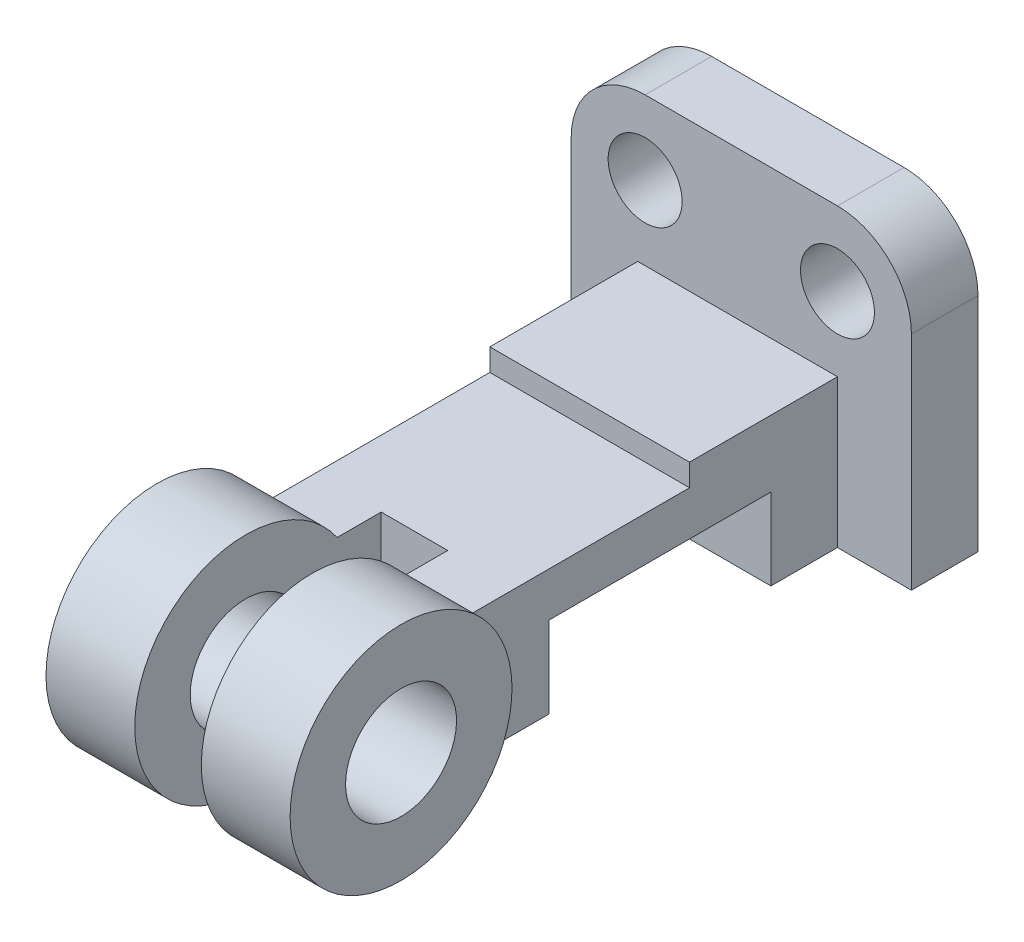
ISO-10303-21;
HEADER;
FILE_DESCRIPTION(('STEP AP214'),'2;1');
FILE_NAME('part.step','',(''),(''),'','','');
FILE_SCHEMA(('AUTOMOTIVE_DESIGN { 1 0 10303 214 1 1 1 1 }'));
ENDSEC;
DATA;
#1=APPLICATION_CONTEXT('core data for automotive mechanical design processes');
#2=APPLICATION_PROTOCOL_DEFINITION('international standard','automotive_design',2000,#1);
#3=PRODUCT_CONTEXT('',#1,'mechanical');
#4=PRODUCT('Part','Part','',(#3));
#5=PRODUCT_RELATED_PRODUCT_CATEGORY('part','',(#4));
#6=PRODUCT_DEFINITION_FORMATION('','',#4);
#7=PRODUCT_DEFINITION_CONTEXT('part definition',#1,'design');
#8=PRODUCT_DEFINITION('design','',#6,#7);
#9=PRODUCT_DEFINITION_SHAPE('','',#8);
#10=(LENGTH_UNIT() NAMED_UNIT(*) SI_UNIT(.MILLI.,.METRE.));
#11=(NAMED_UNIT(*) PLANE_ANGLE_UNIT() SI_UNIT($,.RADIAN.));
#12=(NAMED_UNIT(*) SI_UNIT($,.STERADIAN.) SOLID_ANGLE_UNIT());
#13=UNCERTAINTY_MEASURE_WITH_UNIT(LENGTH_MEASURE(1.E-05),#10,'distance_accuracy_value','');
#14=(GEOMETRIC_REPRESENTATION_CONTEXT(3) GLOBAL_UNCERTAINTY_ASSIGNED_CONTEXT((#13)) GLOBAL_UNIT_ASSIGNED_CONTEXT((#10,
#11,#12)) REPRESENTATION_CONTEXT('',''));
#15=CARTESIAN_POINT('',(0.,0.,0.));
#16=DIRECTION('',(0.,0.,1.));
#17=DIRECTION('',(1.,0.,0.));
#18=AXIS2_PLACEMENT_3D('',#15,#16,#17);
#19=CARTESIAN_POINT('',(78.,17.,142.));
#20=DIRECTION('',(-1.,0.,0.));
#21=DIRECTION('',(0.,-1.,0.));
#22=AXIS2_PLACEMENT_3D('',#19,#20,#21);
#23=CYLINDRICAL_SURFACE('',#22,30.);
#24=CARTESIAN_POINT('',(78.,17.,142.));
#25=DIRECTION('',(1.,0.,0.));
#26=DIRECTION('',(0.,1.,0.));
#27=AXIS2_PLACEMENT_3D('',#24,#25,#26);
#28=CIRCLE('',#27,30.);
#29=CARTESIAN_POINT('',(78.,47.,142.));
#30=VERTEX_POINT('',#29);
#31=EDGE_CURVE('E224',#30,#30,#28,.T.);
#32=ORIENTED_EDGE('',*,*,#31,.F.);
#33=EDGE_LOOP('',(#32));
#34=FACE_BOUND('',#33,.T.);
#35=CARTESIAN_POINT('',(54.,17.,142.));
#36=DIRECTION('',(-1.,0.,0.));
#37=DIRECTION('',(0.,0.,1.));
#38=AXIS2_PLACEMENT_3D('',#35,#36,#37);
#39=CIRCLE('',#38,30.);
#40=CARTESIAN_POINT('',(54.,0.,117.281585811383));
#41=VERTEX_POINT('',#40);
#42=CARTESIAN_POINT('',(54.,34.,117.281585811383));
#43=VERTEX_POINT('',#42);
#44=EDGE_CURVE('E187',#41,#43,#39,.T.);
#45=ORIENTED_EDGE('',*,*,#44,.F.);
#46=DIRECTION('',(-1.,0.,0.));
#47=VECTOR('',#46,1.);
#48=CARTESIAN_POINT('',(78.,0.,117.281585811383));
#49=LINE('',#48,#47);
#50=CARTESIAN_POINT('',(72.,0.,117.281585811383));
#51=VERTEX_POINT('',#50);
#52=EDGE_CURVE('E233',#41,#51,#49,.F.);
#53=ORIENTED_EDGE('',*,*,#52,.T.);
#54=CARTESIAN_POINT('',(72.,17.,142.));
#55=DIRECTION('',(1.,0.,0.));
#56=DIRECTION('',(0.,1.,0.));
#57=AXIS2_PLACEMENT_3D('',#54,#55,#56);
#58=CIRCLE('',#57,30.);
#59=CARTESIAN_POINT('',(72.,34.,117.281585811383));
#60=VERTEX_POINT('',#59);
#61=EDGE_CURVE('E193',#60,#51,#58,.F.);
#62=ORIENTED_EDGE('',*,*,#61,.F.);
#63=DIRECTION('',(-1.,0.,0.));
#64=VECTOR('',#63,1.);
#65=CARTESIAN_POINT('',(78.,34.,117.281585811383));
#66=LINE('',#65,#64);
#67=EDGE_CURVE('E48',#43,#60,#66,.F.);
#68=ORIENTED_EDGE('',*,*,#67,.F.);
#69=EDGE_LOOP('',(#45,#53,#62,#68));
#70=FACE_BOUND('',#69,.T.);
#71=ADVANCED_FACE('F39',(#34,#70),#23,.T.);
#72=CARTESIAN_POINT('',(78.,17.,142.));
#73=DIRECTION('',(-1.,0.,0.));
#74=DIRECTION('',(0.,-1.,0.));
#75=AXIS2_PLACEMENT_3D('',#72,#73,#74);
#76=CYLINDRICAL_SURFACE('',#75,15.);
#77=CARTESIAN_POINT('',(78.,17.,142.));
#78=DIRECTION('',(1.,0.,0.));
#79=DIRECTION('',(0.,1.,0.));
#80=AXIS2_PLACEMENT_3D('',#77,#78,#79);
#81=CIRCLE('',#80,15.);
#82=CARTESIAN_POINT('',(78.,32.,142.));
#83=VERTEX_POINT('',#82);
#84=EDGE_CURVE('E225',#83,#83,#81,.T.);
#85=ORIENTED_EDGE('',*,*,#84,.T.);
#86=EDGE_LOOP('',(#85));
#87=FACE_BOUND('',#86,.T.);
#88=CARTESIAN_POINT('',(54.,17.,142.));
#89=DIRECTION('',(-1.,0.,0.));
#90=DIRECTION('',(0.,0.,1.));
#91=AXIS2_PLACEMENT_3D('',#88,#89,#90);
#92=CIRCLE('',#91,15.);
#93=CARTESIAN_POINT('',(54.,17.,157.));
#94=VERTEX_POINT('',#93);
#95=EDGE_CURVE('E195',#94,#94,#92,.T.);
#96=ORIENTED_EDGE('',*,*,#95,.T.);
#97=EDGE_LOOP('',(#96));
#98=FACE_BOUND('',#97,.T.);
#99=ADVANCED_FACE('F413',(#87,#98),#76,.F.);
#100=CARTESIAN_POINT('',(0.,0.,18.));
#101=DIRECTION('',(0.,1.,0.));
#102=DIRECTION('',(0.,0.,1.));
#103=AXIS2_PLACEMENT_3D('',#100,#101,#102);
#104=PLANE('',#103);
#105=DIRECTION('',(-1.,0.,0.));
#106=VECTOR('',#105,1.);
#107=CARTESIAN_POINT('',(0.,0.,105.372540600415));
#108=LINE('',#107,#106);
#109=CARTESIAN_POINT('',(54.,0.,105.372540600415));
#110=VERTEX_POINT('',#109);
#111=CARTESIAN_POINT('',(36.,0.,105.372540600415));
#112=VERTEX_POINT('',#111);
#113=EDGE_CURVE('E201',#110,#112,#108,.T.);
#114=ORIENTED_EDGE('',*,*,#113,.T.);
#115=DIRECTION('',(0.,0.,1.));
#116=VECTOR('',#115,1.);
#117=CARTESIAN_POINT('',(36.,0.,18.));
#118=LINE('',#117,#116);
#119=CARTESIAN_POINT('',(36.,0.,117.281585811383));
#120=VERTEX_POINT('',#119);
#121=EDGE_CURVE('E210',#112,#120,#118,.T.);
#122=ORIENTED_EDGE('',*,*,#121,.T.);
#123=CARTESIAN_POINT('',(18.,0.,117.281585811383));
#124=VERTEX_POINT('',#123);
#125=EDGE_CURVE('E235',#124,#120,#49,.F.);
#126=ORIENTED_EDGE('',*,*,#125,.F.);
#127=DIRECTION('',(0.,0.,-1.));
#128=VECTOR('',#127,1.);
#129=CARTESIAN_POINT('',(18.,0.,18.));
#130=LINE('',#129,#128);
#131=CARTESIAN_POINT('',(18.,0.,96.));
#132=VERTEX_POINT('',#131);
#133=EDGE_CURVE('E278',#124,#132,#130,.T.);
#134=ORIENTED_EDGE('',*,*,#133,.T.);
#135=DIRECTION('',(1.,0.,0.));
#136=VECTOR('',#135,1.);
#137=CARTESIAN_POINT('',(18.,0.,96.));
#138=LINE('',#137,#136);
#139=CARTESIAN_POINT('',(72.,0.,96.));
#140=VERTEX_POINT('',#139);
#141=EDGE_CURVE('E260',#132,#140,#138,.T.);
#142=ORIENTED_EDGE('',*,*,#141,.T.);
#143=DIRECTION('',(0.,0.,-1.));
#144=VECTOR('',#143,1.);
#145=CARTESIAN_POINT('',(72.,0.,18.));
#146=LINE('',#145,#144);
#147=EDGE_CURVE('E271',#51,#140,#146,.T.);
#148=ORIENTED_EDGE('',*,*,#147,.F.);
#149=ORIENTED_EDGE('',*,*,#52,.F.);
#150=DIRECTION('',(0.,0.,-1.));
#151=VECTOR('',#150,1.);
#152=CARTESIAN_POINT('',(54.,0.,18.));
#153=LINE('',#152,#151);
#154=EDGE_CURVE('E186',#41,#110,#153,.T.);
#155=ORIENTED_EDGE('',*,*,#154,.T.);
#156=EDGE_LOOP('',(#114,#122,#126,#134,#142,#148,#149,#155));
#157=FACE_BOUND('',#156,.T.);
#158=ADVANCED_FACE('F419',(#157),#104,.F.);
#159=CARTESIAN_POINT('',(18.,34.,58.));
#160=DIRECTION('',(0.,1.,0.));
#161=DIRECTION('',(-1.,0.,0.));
#162=AXIS2_PLACEMENT_3D('',#159,#160,#161);
#163=PLANE('',#162);
#164=DIRECTION('',(0.,0.,1.));
#165=VECTOR('',#164,1.);
#166=CARTESIAN_POINT('',(36.,34.,117.281585811383));
#167=LINE('',#166,#165);
#168=CARTESIAN_POINT('',(36.,34.,105.372540600415));
#169=VERTEX_POINT('',#168);
#170=CARTESIAN_POINT('',(36.,34.,117.281585811383));
#171=VERTEX_POINT('',#170);
#172=EDGE_CURVE('E467',#169,#171,#167,.T.);
#173=ORIENTED_EDGE('',*,*,#172,.F.);
#174=DIRECTION('',(-1.,0.,0.));
#175=VECTOR('',#174,1.);
#176=CARTESIAN_POINT('',(54.,34.,105.372540600415));
#177=LINE('',#176,#175);
#178=CARTESIAN_POINT('',(54.,34.,105.372540600415));
#179=VERTEX_POINT('',#178);
#180=EDGE_CURVE('E181',#179,#169,#177,.T.);
#181=ORIENTED_EDGE('',*,*,#180,.F.);
#182=DIRECTION('',(0.,0.,-1.));
#183=VECTOR('',#182,1.);
#184=CARTESIAN_POINT('',(54.,34.,117.281585811383));
#185=LINE('',#184,#183);
#186=EDGE_CURVE('E176',#43,#179,#185,.T.);
#187=ORIENTED_EDGE('',*,*,#186,.F.);
#188=ORIENTED_EDGE('',*,*,#67,.T.);
#189=DIRECTION('',(0.,0.,1.));
#190=VECTOR('',#189,1.);
#191=CARTESIAN_POINT('',(72.,34.,58.));
#192=LINE('',#191,#190);
#193=CARTESIAN_POINT('',(72.,34.,58.));
#194=VERTEX_POINT('',#193);
#195=EDGE_CURVE('E251',#194,#60,#192,.T.);
#196=ORIENTED_EDGE('',*,*,#195,.F.);
#197=DIRECTION('',(1.,0.,0.));
#198=VECTOR('',#197,1.);
#199=CARTESIAN_POINT('',(18.,34.,58.));
#200=LINE('',#199,#198);
#201=CARTESIAN_POINT('',(18.,34.,58.));
#202=VERTEX_POINT('',#201);
#203=EDGE_CURVE('E265',#202,#194,#200,.T.);
#204=ORIENTED_EDGE('',*,*,#203,.F.);
#205=DIRECTION('',(0.,0.,1.));
#206=VECTOR('',#205,1.);
#207=CARTESIAN_POINT('',(18.,34.,58.));
#208=LINE('',#207,#206);
#209=CARTESIAN_POINT('',(18.,34.,117.281585811383));
#210=VERTEX_POINT('',#209);
#211=EDGE_CURVE('E263',#202,#210,#208,.T.);
#212=ORIENTED_EDGE('',*,*,#211,.T.);
#213=EDGE_CURVE('E11',#210,#171,#66,.F.);
#214=ORIENTED_EDGE('',*,*,#213,.T.);
#215=EDGE_LOOP('',(#173,#181,#187,#188,#196,#204,#212,#214));
#216=FACE_BOUND('',#215,.T.);
#217=ADVANCED_FACE('F177',(#216),#163,.T.);
#218=CARTESIAN_POINT('',(72.,0.,36.));
#219=VERTEX_POINT('',#218);
#220=CARTESIAN_POINT('',(72.,0.,18.));
#221=VERTEX_POINT('',#220);
#222=EDGE_CURVE('E289',#219,#221,#146,.T.);
#223=ORIENTED_EDGE('',*,*,#222,.F.);
#224=DIRECTION('',(1.,0.,0.));
#225=VECTOR('',#224,1.);
#226=CARTESIAN_POINT('',(18.,0.,36.));
#227=LINE('',#226,#225);
#228=CARTESIAN_POINT('',(18.,0.,36.));
#229=VERTEX_POINT('',#228);
#230=EDGE_CURVE('E253',#229,#219,#227,.T.);
#231=ORIENTED_EDGE('',*,*,#230,.F.);
#232=CARTESIAN_POINT('',(18.,0.,18.));
#233=VERTEX_POINT('',#232);
#234=EDGE_CURVE('E276',#229,#233,#130,.T.);
#235=ORIENTED_EDGE('',*,*,#234,.T.);
#236=DIRECTION('',(1.,0.,0.));
#237=VECTOR('',#236,1.);
#238=CARTESIAN_POINT('',(0.,0.,18.));
#239=LINE('',#238,#237);
#240=CARTESIAN_POINT('',(0.,0.,18.));
#241=VERTEX_POINT('',#240);
#242=EDGE_CURVE('E313',#241,#233,#239,.T.);
#243=ORIENTED_EDGE('',*,*,#242,.F.);
#244=DIRECTION('',(0.,0.,-1.));
#245=VECTOR('',#244,1.);
#246=CARTESIAN_POINT('',(0.,0.,18.));
#247=LINE('',#246,#245);
#248=CARTESIAN_POINT('',(0.,0.,0.));
#249=VERTEX_POINT('',#248);
#250=EDGE_CURVE('E199',#241,#249,#247,.T.);
#251=ORIENTED_EDGE('',*,*,#250,.T.);
#252=DIRECTION('',(1.,0.,0.));
#253=VECTOR('',#252,1.);
#254=CARTESIAN_POINT('',(0.,0.,0.));
#255=LINE('',#254,#253);
#256=CARTESIAN_POINT('',(92.,0.,0.));
#257=VERTEX_POINT('',#256);
#258=EDGE_CURVE('E327',#249,#257,#255,.T.);
#259=ORIENTED_EDGE('',*,*,#258,.T.);
#260=DIRECTION('',(0.,0.,-1.));
#261=VECTOR('',#260,1.);
#262=CARTESIAN_POINT('',(92.,0.,18.));
#263=LINE('',#262,#261);
#264=CARTESIAN_POINT('',(92.,0.,18.));
#265=VERTEX_POINT('',#264);
#266=EDGE_CURVE('E200',#265,#257,#263,.T.);
#267=ORIENTED_EDGE('',*,*,#266,.F.);
#268=EDGE_CURVE('E315',#221,#265,#239,.T.);
#269=ORIENTED_EDGE('',*,*,#268,.F.);
#270=EDGE_LOOP('',(#223,#231,#235,#243,#251,#259,#267,#269));
#271=FACE_BOUND('',#270,.T.);
#272=ADVANCED_FACE('F380',(#271),#104,.F.);
#273=CARTESIAN_POINT('',(18.,0.,58.));
#274=DIRECTION('',(0.,0.,1.));
#275=DIRECTION('',(1.,0.,0.));
#276=AXIS2_PLACEMENT_3D('',#273,#274,#275);
#277=PLANE('',#276);
#278=DIRECTION('',(0.,-1.,0.));
#279=VECTOR('',#278,1.);
#280=CARTESIAN_POINT('',(18.,0.,58.));
#281=LINE('',#280,#279);
#282=CARTESIAN_POINT('',(18.,40.,58.));
#283=VERTEX_POINT('',#282);
#284=EDGE_CURVE('E277',#283,#202,#281,.T.);
#285=ORIENTED_EDGE('',*,*,#284,.T.);
#286=ORIENTED_EDGE('',*,*,#203,.T.);
#287=DIRECTION('',(0.,-1.,0.));
#288=VECTOR('',#287,1.);
#289=CARTESIAN_POINT('',(72.,0.,58.));
#290=LINE('',#289,#288);
#291=CARTESIAN_POINT('',(72.,40.,58.));
#292=VERTEX_POINT('',#291);
#293=EDGE_CURVE('E290',#292,#194,#290,.T.);
#294=ORIENTED_EDGE('',*,*,#293,.F.);
#295=DIRECTION('',(1.,0.,0.));
#296=VECTOR('',#295,1.);
#297=CARTESIAN_POINT('',(18.,40.,58.));
#298=LINE('',#297,#296);
#299=EDGE_CURVE('E292',#283,#292,#298,.T.);
#300=ORIENTED_EDGE('',*,*,#299,.F.);
#301=EDGE_LOOP('',(#285,#286,#294,#300));
#302=FACE_BOUND('',#301,.T.);
#303=ADVANCED_FACE('F471',(#302),#277,.T.);
#304=CARTESIAN_POINT('',(20.,60.,18.));
#305=DIRECTION('',(0.,0.,-1.));
#306=DIRECTION('',(-1.,0.,0.));
#307=AXIS2_PLACEMENT_3D('',#304,#305,#306);
#308=PLANE('',#307);
#309=CARTESIAN_POINT('',(72.,60.,18.));
#310=DIRECTION('',(0.,0.,1.));
#311=DIRECTION('',(1.,0.,0.));
#312=AXIS2_PLACEMENT_3D('',#309,#310,#311);
#313=CIRCLE('',#312,9.99999999999999);
#314=CARTESIAN_POINT('',(82.,60.,18.));
#315=VERTEX_POINT('',#314);
#316=EDGE_CURVE('E300',#315,#315,#313,.T.);
#317=ORIENTED_EDGE('',*,*,#316,.F.);
#318=EDGE_LOOP('',(#317));
#319=FACE_BOUND('',#318,.T.);
#320=CARTESIAN_POINT('',(20.,60.,18.));
#321=DIRECTION('',(0.,0.,1.));
#322=DIRECTION('',(1.,0.,0.));
#323=AXIS2_PLACEMENT_3D('',#320,#321,#322);
#324=CIRCLE('',#323,10.);
#325=CARTESIAN_POINT('',(30.,60.,18.));
#326=VERTEX_POINT('',#325);
#327=EDGE_CURVE('E303',#326,#326,#324,.T.);
#328=ORIENTED_EDGE('',*,*,#327,.F.);
#329=EDGE_LOOP('',(#328));
#330=FACE_BOUND('',#329,.T.);
#331=DIRECTION('',(0.,1.,0.));
#332=VECTOR('',#331,1.);
#333=CARTESIAN_POINT('',(72.,0.,18.));
#334=LINE('',#333,#332);
#335=CARTESIAN_POINT('',(72.,40.,18.));
#336=VERTEX_POINT('',#335);
#337=EDGE_CURVE('E266',#221,#336,#334,.T.);
#338=ORIENTED_EDGE('',*,*,#337,.F.);
#339=ORIENTED_EDGE('',*,*,#268,.T.);
#340=DIRECTION('',(0.,1.,0.));
#341=VECTOR('',#340,1.);
#342=CARTESIAN_POINT('',(92.,0.,18.));
#343=LINE('',#342,#341);
#344=CARTESIAN_POINT('',(92.,59.9999999999999,18.));
#345=VERTEX_POINT('',#344);
#346=EDGE_CURVE('E320',#265,#345,#343,.T.);
#347=ORIENTED_EDGE('',*,*,#346,.T.);
#348=CARTESIAN_POINT('',(72.,60.,18.));
#349=DIRECTION('',(0.,0.,1.));
#350=DIRECTION('',(-1.,0.,0.));
#351=AXIS2_PLACEMENT_3D('',#348,#349,#350);
#352=CIRCLE('',#351,20.);
#353=CARTESIAN_POINT('',(71.9999999999998,80.,18.));
#354=VERTEX_POINT('',#353);
#355=EDGE_CURVE('E316',#345,#354,#352,.T.);
#356=ORIENTED_EDGE('',*,*,#355,.T.);
#357=DIRECTION('',(-1.,0.,0.));
#358=VECTOR('',#357,1.);
#359=CARTESIAN_POINT('',(20.0000000000001,80.,18.));
#360=LINE('',#359,#358);
#361=CARTESIAN_POINT('',(20.0000000000001,80.,18.));
#362=VERTEX_POINT('',#361);
#363=EDGE_CURVE('E322',#354,#362,#360,.T.);
#364=ORIENTED_EDGE('',*,*,#363,.T.);
#365=CARTESIAN_POINT('',(20.,60.,18.));
#366=DIRECTION('',(0.,0.,1.));
#367=DIRECTION('',(-1.,0.,0.));
#368=AXIS2_PLACEMENT_3D('',#365,#366,#367);
#369=CIRCLE('',#368,20.);
#370=CARTESIAN_POINT('',(0.,59.9999999999999,18.));
#371=VERTEX_POINT('',#370);
#372=EDGE_CURVE('E324',#362,#371,#369,.T.);
#373=ORIENTED_EDGE('',*,*,#372,.T.);
#374=DIRECTION('',(0.,-1.,0.));
#375=VECTOR('',#374,1.);
#376=CARTESIAN_POINT('',(0.,0.,18.));
#377=LINE('',#376,#375);
#378=EDGE_CURVE('E307',#371,#241,#377,.T.);
#379=ORIENTED_EDGE('',*,*,#378,.T.);
#380=ORIENTED_EDGE('',*,*,#242,.T.);
#381=DIRECTION('',(0.,1.,0.));
#382=VECTOR('',#381,1.);
#383=CARTESIAN_POINT('',(18.,0.,18.));
#384=LINE('',#383,#382);
#385=CARTESIAN_POINT('',(18.,40.,18.));
#386=VERTEX_POINT('',#385);
#387=EDGE_CURVE('E267',#233,#386,#384,.T.);
#388=ORIENTED_EDGE('',*,*,#387,.T.);
#389=DIRECTION('',(1.,0.,0.));
#390=VECTOR('',#389,1.);
#391=CARTESIAN_POINT('',(18.,40.,18.));
#392=LINE('',#391,#390);
#393=EDGE_CURVE('E284',#386,#336,#392,.T.);
#394=ORIENTED_EDGE('',*,*,#393,.T.);
#395=EDGE_LOOP('',(#338,#339,#347,#356,#364,#373,#379,#380,#388,#394));
#396=FACE_BOUND('',#395,.T.);
#397=ADVANCED_FACE('F372',(#319,#330,#396),#308,.F.);
#398=CARTESIAN_POINT('',(20.,60.,0.));
#399=DIRECTION('',(0.,0.,-1.));
#400=DIRECTION('',(-1.,0.,0.));
#401=AXIS2_PLACEMENT_3D('',#398,#399,#400);
#402=PLANE('',#401);
#403=CARTESIAN_POINT('',(20.,60.,0.));
#404=DIRECTION('',(0.,0.,1.));
#405=DIRECTION('',(1.,0.,0.));
#406=AXIS2_PLACEMENT_3D('',#403,#404,#405);
#407=CIRCLE('',#406,10.);
#408=CARTESIAN_POINT('',(30.,60.,0.));
#409=VERTEX_POINT('',#408);
#410=EDGE_CURVE('E297',#409,#409,#407,.T.);
#411=ORIENTED_EDGE('',*,*,#410,.T.);
#412=EDGE_LOOP('',(#411));
#413=FACE_BOUND('',#412,.T.);
#414=DIRECTION('',(0.,-1.,0.));
#415=VECTOR('',#414,1.);
#416=CARTESIAN_POINT('',(0.,0.,0.));
#417=LINE('',#416,#415);
#418=CARTESIAN_POINT('',(0.,59.9999999999999,0.));
#419=VERTEX_POINT('',#418);
#420=EDGE_CURVE('E306',#419,#249,#417,.T.);
#421=ORIENTED_EDGE('',*,*,#420,.F.);
#422=CARTESIAN_POINT('',(20.,60.,0.));
#423=DIRECTION('',(0.,0.,1.));
#424=DIRECTION('',(-1.,0.,0.));
#425=AXIS2_PLACEMENT_3D('',#422,#423,#424);
#426=CIRCLE('',#425,20.);
#427=CARTESIAN_POINT('',(20.0000000000001,80.,0.));
#428=VERTEX_POINT('',#427);
#429=EDGE_CURVE('E312',#428,#419,#426,.T.);
#430=ORIENTED_EDGE('',*,*,#429,.F.);
#431=DIRECTION('',(-1.,0.,0.));
#432=VECTOR('',#431,1.);
#433=CARTESIAN_POINT('',(20.0000000000001,80.,0.));
#434=LINE('',#433,#432);
#435=CARTESIAN_POINT('',(71.9999999999998,80.,0.));
#436=VERTEX_POINT('',#435);
#437=EDGE_CURVE('E332',#436,#428,#434,.T.);
#438=ORIENTED_EDGE('',*,*,#437,.F.);
#439=CARTESIAN_POINT('',(72.,60.,0.));
#440=DIRECTION('',(0.,0.,1.));
#441=DIRECTION('',(-1.,0.,0.));
#442=AXIS2_PLACEMENT_3D('',#439,#440,#441);
#443=CIRCLE('',#442,20.);
#444=CARTESIAN_POINT('',(92.,59.9999999999999,0.));
#445=VERTEX_POINT('',#444);
#446=EDGE_CURVE('E335',#445,#436,#443,.T.);
#447=ORIENTED_EDGE('',*,*,#446,.F.);
#448=DIRECTION('',(0.,1.,0.));
#449=VECTOR('',#448,1.);
#450=CARTESIAN_POINT('',(92.,0.,0.));
#451=LINE('',#450,#449);
#452=EDGE_CURVE('E326',#257,#445,#451,.T.);
#453=ORIENTED_EDGE('',*,*,#452,.F.);
#454=ORIENTED_EDGE('',*,*,#258,.F.);
#455=EDGE_LOOP('',(#421,#430,#438,#447,#453,#454));
#456=FACE_BOUND('',#455,.T.);
#457=CARTESIAN_POINT('',(72.,60.,0.));
#458=DIRECTION('',(0.,0.,1.));
#459=DIRECTION('',(1.,0.,0.));
#460=AXIS2_PLACEMENT_3D('',#457,#458,#459);
#461=CIRCLE('',#460,9.99999999999999);
#462=CARTESIAN_POINT('',(82.,60.,0.));
#463=VERTEX_POINT('',#462);
#464=EDGE_CURVE('E295',#463,#463,#461,.T.);
#465=ORIENTED_EDGE('',*,*,#464,.T.);
#466=EDGE_LOOP('',(#465));
#467=FACE_BOUND('',#466,.T.);
#468=ADVANCED_FACE('F360',(#413,#456,#467),#402,.T.);
#469=CARTESIAN_POINT('',(0.,0.,18.));
#470=DIRECTION('',(1.,0.,0.));
#471=DIRECTION('',(0.,1.,0.));
#472=AXIS2_PLACEMENT_3D('',#469,#470,#471);
#473=PLANE('',#472);
#474=ORIENTED_EDGE('',*,*,#420,.T.);
#475=ORIENTED_EDGE('',*,*,#250,.F.);
#476=ORIENTED_EDGE('',*,*,#378,.F.);
#477=DIRECTION('',(0.,0.,-1.));
#478=VECTOR('',#477,1.);
#479=CARTESIAN_POINT('',(0.,59.9999999999999,18.));
#480=LINE('',#479,#478);
#481=EDGE_CURVE('E323',#371,#419,#480,.T.);
#482=ORIENTED_EDGE('',*,*,#481,.T.);
#483=EDGE_LOOP('',(#474,#475,#476,#482));
#484=FACE_BOUND('',#483,.T.);
#485=ADVANCED_FACE('F41',(#484),#473,.F.);
#486=CARTESIAN_POINT('',(92.,0.,18.));
#487=DIRECTION('',(-1.,0.,0.));
#488=DIRECTION('',(0.,-1.,0.));
#489=AXIS2_PLACEMENT_3D('',#486,#487,#488);
#490=PLANE('',#489);
#491=ORIENTED_EDGE('',*,*,#452,.T.);
#492=DIRECTION('',(0.,0.,-1.));
#493=VECTOR('',#492,1.);
#494=CARTESIAN_POINT('',(92.,59.9999999999999,18.));
#495=LINE('',#494,#493);
#496=EDGE_CURVE('E343',#345,#445,#495,.T.);
#497=ORIENTED_EDGE('',*,*,#496,.F.);
#498=ORIENTED_EDGE('',*,*,#346,.F.);
#499=ORIENTED_EDGE('',*,*,#266,.T.);
#500=EDGE_LOOP('',(#491,#497,#498,#499));
#501=FACE_BOUND('',#500,.T.);
#502=ADVANCED_FACE('F355',(#501),#490,.F.);
#503=CARTESIAN_POINT('',(72.,60.,18.));
#504=DIRECTION('',(0.,0.,-1.));
#505=DIRECTION('',(-1.,0.,0.));
#506=AXIS2_PLACEMENT_3D('',#503,#504,#505);
#507=CYLINDRICAL_SURFACE('',#506,20.);
#508=ORIENTED_EDGE('',*,*,#446,.T.);
#509=DIRECTION('',(0.,0.,-1.));
#510=VECTOR('',#509,1.);
#511=CARTESIAN_POINT('',(71.9999999999998,80.,18.));
#512=LINE('',#511,#510);
#513=EDGE_CURVE('E345',#354,#436,#512,.T.);
#514=ORIENTED_EDGE('',*,*,#513,.F.);
#515=ORIENTED_EDGE('',*,*,#355,.F.);
#516=ORIENTED_EDGE('',*,*,#496,.T.);
#517=EDGE_LOOP('',(#508,#514,#515,#516));
#518=FACE_BOUND('',#517,.T.);
#519=ADVANCED_FACE('F362',(#518),#507,.T.);
#520=CARTESIAN_POINT('',(20.0000000000001,80.,18.));
#521=DIRECTION('',(0.,-1.,0.));
#522=DIRECTION('',(0.,0.,-1.));
#523=AXIS2_PLACEMENT_3D('',#520,#521,#522);
#524=PLANE('',#523);
#525=ORIENTED_EDGE('',*,*,#437,.T.);
#526=DIRECTION('',(0.,0.,-1.));
#527=VECTOR('',#526,1.);
#528=CARTESIAN_POINT('',(20.0000000000001,80.,18.));
#529=LINE('',#528,#527);
#530=EDGE_CURVE('E339',#362,#428,#529,.T.);
#531=ORIENTED_EDGE('',*,*,#530,.F.);
#532=ORIENTED_EDGE('',*,*,#363,.F.);
#533=ORIENTED_EDGE('',*,*,#513,.T.);
#534=EDGE_LOOP('',(#525,#531,#532,#533));
#535=FACE_BOUND('',#534,.T.);
#536=ADVANCED_FACE('F367',(#535),#524,.F.);
#537=CARTESIAN_POINT('',(20.,60.,18.));
#538=DIRECTION('',(0.,0.,-1.));
#539=DIRECTION('',(-1.,0.,0.));
#540=AXIS2_PLACEMENT_3D('',#537,#538,#539);
#541=CYLINDRICAL_SURFACE('',#540,20.);
#542=ORIENTED_EDGE('',*,*,#429,.T.);
#543=ORIENTED_EDGE('',*,*,#481,.F.);
#544=ORIENTED_EDGE('',*,*,#372,.F.);
#545=ORIENTED_EDGE('',*,*,#530,.T.);
#546=EDGE_LOOP('',(#542,#543,#544,#545));
#547=FACE_BOUND('',#546,.T.);
#548=ADVANCED_FACE('F400',(#547),#541,.T.);
#549=CARTESIAN_POINT('',(20.,60.,18.));
#550=DIRECTION('',(0.,0.,-1.));
#551=DIRECTION('',(-1.,0.,0.));
#552=AXIS2_PLACEMENT_3D('',#549,#550,#551);
#553=CYLINDRICAL_SURFACE('',#552,10.);
#554=ORIENTED_EDGE('',*,*,#327,.T.);
#555=EDGE_LOOP('',(#554));
#556=FACE_BOUND('',#555,.T.);
#557=ORIENTED_EDGE('',*,*,#410,.F.);
#558=EDGE_LOOP('',(#557));
#559=FACE_BOUND('',#558,.T.);
#560=ADVANCED_FACE('F397',(#556,#559),#553,.F.);
#561=CARTESIAN_POINT('',(72.,60.,18.));
#562=DIRECTION('',(0.,0.,-1.));
#563=DIRECTION('',(-1.,0.,0.));
#564=AXIS2_PLACEMENT_3D('',#561,#562,#563);
#565=CYLINDRICAL_SURFACE('',#564,9.99999999999999);
#566=ORIENTED_EDGE('',*,*,#316,.T.);
#567=EDGE_LOOP('',(#566));
#568=FACE_BOUND('',#567,.T.);
#569=ORIENTED_EDGE('',*,*,#464,.F.);
#570=EDGE_LOOP('',(#569));
#571=FACE_BOUND('',#570,.T.);
#572=ADVANCED_FACE('F403',(#568,#571),#565,.F.);
#573=CARTESIAN_POINT('',(18.,40.,18.));
#574=DIRECTION('',(0.,1.,0.));
#575=DIRECTION('',(-1.,0.,0.));
#576=AXIS2_PLACEMENT_3D('',#573,#574,#575);
#577=PLANE('',#576);
#578=DIRECTION('',(0.,0.,1.));
#579=VECTOR('',#578,1.);
#580=CARTESIAN_POINT('',(72.,40.,18.));
#581=LINE('',#580,#579);
#582=EDGE_CURVE('E285',#336,#292,#581,.T.);
#583=ORIENTED_EDGE('',*,*,#582,.F.);
#584=ORIENTED_EDGE('',*,*,#393,.F.);
#585=DIRECTION('',(0.,0.,1.));
#586=VECTOR('',#585,1.);
#587=CARTESIAN_POINT('',(18.,40.,18.));
#588=LINE('',#587,#586);
#589=EDGE_CURVE('E275',#386,#283,#588,.T.);
#590=ORIENTED_EDGE('',*,*,#589,.T.);
#591=ORIENTED_EDGE('',*,*,#299,.T.);
#592=EDGE_LOOP('',(#583,#584,#590,#591));
#593=FACE_BOUND('',#592,.T.);
#594=ADVANCED_FACE('F479',(#593),#577,.T.);
#595=CARTESIAN_POINT('',(18.,0.,0.));
#596=DIRECTION('',(1.,0.,0.));
#597=DIRECTION('',(0.,1.,0.));
#598=AXIS2_PLACEMENT_3D('',#595,#596,#597);
#599=PLANE('',#598);
#600=CARTESIAN_POINT('',(18.,17.,142.));
#601=DIRECTION('',(1.,0.,0.));
#602=DIRECTION('',(0.,1.,0.));
#603=AXIS2_PLACEMENT_3D('',#600,#601,#602);
#604=CIRCLE('',#603,30.);
#605=EDGE_CURVE('E230',#210,#124,#604,.F.);
#606=ORIENTED_EDGE('',*,*,#605,.F.);
#607=ORIENTED_EDGE('',*,*,#211,.F.);
#608=ORIENTED_EDGE('',*,*,#284,.F.);
#609=ORIENTED_EDGE('',*,*,#589,.F.);
#610=ORIENTED_EDGE('',*,*,#387,.F.);
#611=ORIENTED_EDGE('',*,*,#234,.F.);
#612=DIRECTION('',(0.,1.,0.));
#613=VECTOR('',#612,1.);
#614=CARTESIAN_POINT('',(18.,0.,36.));
#615=LINE('',#614,#613);
#616=CARTESIAN_POINT('',(18.,22.,36.));
#617=VERTEX_POINT('',#616);
#618=EDGE_CURVE('E245',#229,#617,#615,.T.);
#619=ORIENTED_EDGE('',*,*,#618,.T.);
#620=DIRECTION('',(0.,0.,1.));
#621=VECTOR('',#620,1.);
#622=CARTESIAN_POINT('',(18.,22.,0.));
#623=LINE('',#622,#621);
#624=CARTESIAN_POINT('',(18.,22.,96.));
#625=VERTEX_POINT('',#624);
#626=EDGE_CURVE('E232',#617,#625,#623,.T.);
#627=ORIENTED_EDGE('',*,*,#626,.T.);
#628=DIRECTION('',(0.,-1.,0.));
#629=VECTOR('',#628,1.);
#630=CARTESIAN_POINT('',(18.,0.,96.));
#631=LINE('',#630,#629);
#632=EDGE_CURVE('E238',#625,#132,#631,.T.);
#633=ORIENTED_EDGE('',*,*,#632,.T.);
#634=ORIENTED_EDGE('',*,*,#133,.F.);
#635=EDGE_LOOP('',(#606,#607,#608,#609,#610,#611,#619,#627,#633,#634));
#636=FACE_BOUND('',#635,.T.);
#637=ADVANCED_FACE('F388',(#636),#599,.F.);
#638=CARTESIAN_POINT('',(72.,0.,0.));
#639=DIRECTION('',(1.,0.,0.));
#640=DIRECTION('',(0.,1.,0.));
#641=AXIS2_PLACEMENT_3D('',#638,#639,#640);
#642=PLANE('',#641);
#643=ORIENTED_EDGE('',*,*,#195,.T.);
#644=ORIENTED_EDGE('',*,*,#61,.T.);
#645=ORIENTED_EDGE('',*,*,#147,.T.);
#646=DIRECTION('',(0.,-1.,0.));
#647=VECTOR('',#646,1.);
#648=CARTESIAN_POINT('',(72.,0.,96.));
#649=LINE('',#648,#647);
#650=CARTESIAN_POINT('',(72.,22.,96.));
#651=VERTEX_POINT('',#650);
#652=EDGE_CURVE('E250',#651,#140,#649,.T.);
#653=ORIENTED_EDGE('',*,*,#652,.F.);
#654=DIRECTION('',(0.,0.,1.));
#655=VECTOR('',#654,1.);
#656=CARTESIAN_POINT('',(72.,22.,0.));
#657=LINE('',#656,#655);
#658=CARTESIAN_POINT('',(72.,22.,36.));
#659=VERTEX_POINT('',#658);
#660=EDGE_CURVE('E64',#659,#651,#657,.T.);
#661=ORIENTED_EDGE('',*,*,#660,.F.);
#662=DIRECTION('',(0.,1.,0.));
#663=VECTOR('',#662,1.);
#664=CARTESIAN_POINT('',(72.,0.,36.));
#665=LINE('',#664,#663);
#666=EDGE_CURVE('E237',#219,#659,#665,.T.);
#667=ORIENTED_EDGE('',*,*,#666,.F.);
#668=ORIENTED_EDGE('',*,*,#222,.T.);
#669=ORIENTED_EDGE('',*,*,#337,.T.);
#670=ORIENTED_EDGE('',*,*,#582,.T.);
#671=ORIENTED_EDGE('',*,*,#293,.T.);
#672=EDGE_LOOP('',(#643,#644,#645,#653,#661,#667,#668,#669,#670,#671));
#673=FACE_BOUND('',#672,.T.);
#674=ADVANCED_FACE('F385',(#673),#642,.T.);
#675=CARTESIAN_POINT('',(18.,22.,0.));
#676=DIRECTION('',(0.,1.,0.));
#677=DIRECTION('',(-1.,0.,0.));
#678=AXIS2_PLACEMENT_3D('',#675,#676,#677);
#679=PLANE('',#678);
#680=ORIENTED_EDGE('',*,*,#660,.T.);
#681=DIRECTION('',(1.,0.,0.));
#682=VECTOR('',#681,1.);
#683=CARTESIAN_POINT('',(18.,22.,96.));
#684=LINE('',#683,#682);
#685=EDGE_CURVE('E244',#625,#651,#684,.T.);
#686=ORIENTED_EDGE('',*,*,#685,.F.);
#687=ORIENTED_EDGE('',*,*,#626,.F.);
#688=DIRECTION('',(1.,0.,0.));
#689=VECTOR('',#688,1.);
#690=CARTESIAN_POINT('',(18.,22.,36.));
#691=LINE('',#690,#689);
#692=EDGE_CURVE('E255',#617,#659,#691,.T.);
#693=ORIENTED_EDGE('',*,*,#692,.T.);
#694=EDGE_LOOP('',(#680,#686,#687,#693));
#695=FACE_BOUND('',#694,.T.);
#696=ADVANCED_FACE('F531',(#695),#679,.F.);
#697=CARTESIAN_POINT('',(18.,0.,36.));
#698=DIRECTION('',(0.,0.,-1.));
#699=DIRECTION('',(-1.,0.,0.));
#700=AXIS2_PLACEMENT_3D('',#697,#698,#699);
#701=PLANE('',#700);
#702=ORIENTED_EDGE('',*,*,#666,.T.);
#703=ORIENTED_EDGE('',*,*,#692,.F.);
#704=ORIENTED_EDGE('',*,*,#618,.F.);
#705=ORIENTED_EDGE('',*,*,#230,.T.);
#706=EDGE_LOOP('',(#702,#703,#704,#705));
#707=FACE_BOUND('',#706,.T.);
#708=ADVANCED_FACE('F387',(#707),#701,.F.);
#709=CARTESIAN_POINT('',(18.,0.,96.));
#710=DIRECTION('',(0.,0.,1.));
#711=DIRECTION('',(1.,0.,0.));
#712=AXIS2_PLACEMENT_3D('',#709,#710,#711);
#713=PLANE('',#712);
#714=ORIENTED_EDGE('',*,*,#652,.T.);
#715=ORIENTED_EDGE('',*,*,#141,.F.);
#716=ORIENTED_EDGE('',*,*,#632,.F.);
#717=ORIENTED_EDGE('',*,*,#685,.T.);
#718=EDGE_LOOP('',(#714,#715,#716,#717));
#719=FACE_BOUND('',#718,.T.);
#720=ADVANCED_FACE('F429',(#719),#713,.F.);
#721=ORIENTED_EDGE('',*,*,#125,.T.);
#722=CARTESIAN_POINT('',(36.,17.,142.));
#723=DIRECTION('',(-1.,0.,0.));
#724=DIRECTION('',(0.,0.,1.));
#725=AXIS2_PLACEMENT_3D('',#722,#723,#724);
#726=CIRCLE('',#725,30.);
#727=EDGE_CURVE('E214',#120,#171,#726,.T.);
#728=ORIENTED_EDGE('',*,*,#727,.T.);
#729=ORIENTED_EDGE('',*,*,#213,.F.);
#730=ORIENTED_EDGE('',*,*,#605,.T.);
#731=EDGE_LOOP('',(#721,#728,#729,#730));
#732=FACE_BOUND('',#731,.T.);
#733=CARTESIAN_POINT('',(12.,17.,142.));
#734=DIRECTION('',(1.,0.,0.));
#735=DIRECTION('',(0.,1.,0.));
#736=AXIS2_PLACEMENT_3D('',#733,#734,#735);
#737=CIRCLE('',#736,30.);
#738=CARTESIAN_POINT('',(12.,47.,142.));
#739=VERTEX_POINT('',#738);
#740=EDGE_CURVE('E220',#739,#739,#737,.T.);
#741=ORIENTED_EDGE('',*,*,#740,.T.);
#742=EDGE_LOOP('',(#741));
#743=FACE_BOUND('',#742,.T.);
#744=ADVANCED_FACE('F415',(#732,#743),#23,.T.);
#745=CARTESIAN_POINT('',(78.,17.,142.));
#746=DIRECTION('',(1.,0.,0.));
#747=DIRECTION('',(0.,1.,0.));
#748=AXIS2_PLACEMENT_3D('',#745,#746,#747);
#749=PLANE('',#748);
#750=ORIENTED_EDGE('',*,*,#31,.T.);
#751=EDGE_LOOP('',(#750));
#752=FACE_BOUND('',#751,.T.);
#753=ORIENTED_EDGE('',*,*,#84,.F.);
#754=EDGE_LOOP('',(#753));
#755=FACE_BOUND('',#754,.T.);
#756=ADVANCED_FACE('F426',(#752,#755),#749,.T.);
#757=CARTESIAN_POINT('',(36.,17.,142.));
#758=DIRECTION('',(-1.,0.,0.));
#759=DIRECTION('',(0.,0.,1.));
#760=AXIS2_PLACEMENT_3D('',#757,#758,#759);
#761=CIRCLE('',#760,15.);
#762=CARTESIAN_POINT('',(36.,17.,157.));
#763=VERTEX_POINT('',#762);
#764=EDGE_CURVE('E43',#763,#763,#761,.T.);
#765=ORIENTED_EDGE('',*,*,#764,.F.);
#766=EDGE_LOOP('',(#765));
#767=FACE_BOUND('',#766,.T.);
#768=CARTESIAN_POINT('',(12.,17.,142.));
#769=DIRECTION('',(1.,0.,0.));
#770=DIRECTION('',(0.,1.,0.));
#771=AXIS2_PLACEMENT_3D('',#768,#769,#770);
#772=CIRCLE('',#771,15.);
#773=CARTESIAN_POINT('',(12.,32.,142.));
#774=VERTEX_POINT('',#773);
#775=EDGE_CURVE('E218',#774,#774,#772,.T.);
#776=ORIENTED_EDGE('',*,*,#775,.F.);
#777=EDGE_LOOP('',(#776));
#778=FACE_BOUND('',#777,.T.);
#779=ADVANCED_FACE('F421',(#767,#778),#76,.F.);
#780=CARTESIAN_POINT('',(12.,17.,142.));
#781=DIRECTION('',(1.,0.,0.));
#782=DIRECTION('',(0.,1.,0.));
#783=AXIS2_PLACEMENT_3D('',#780,#781,#782);
#784=PLANE('',#783);
#785=ORIENTED_EDGE('',*,*,#775,.T.);
#786=EDGE_LOOP('',(#785));
#787=FACE_BOUND('',#786,.T.);
#788=ORIENTED_EDGE('',*,*,#740,.F.);
#789=EDGE_LOOP('',(#788));
#790=FACE_BOUND('',#789,.T.);
#791=ADVANCED_FACE('F443',(#787,#790),#784,.F.);
#792=CARTESIAN_POINT('',(36.,-13.,117.281585811383));
#793=DIRECTION('',(-1.,0.,0.));
#794=DIRECTION('',(0.,0.,1.));
#795=AXIS2_PLACEMENT_3D('',#792,#793,#794);
#796=PLANE('',#795);
#797=ORIENTED_EDGE('',*,*,#764,.T.);
#798=EDGE_LOOP('',(#797));
#799=FACE_BOUND('',#798,.T.);
#800=ORIENTED_EDGE('',*,*,#727,.F.);
#801=ORIENTED_EDGE('',*,*,#121,.F.);
#802=DIRECTION('',(0.,1.,0.));
#803=VECTOR('',#802,1.);
#804=CARTESIAN_POINT('',(36.,-13.,105.372540600415));
#805=LINE('',#804,#803);
#806=EDGE_CURVE('E464',#112,#169,#805,.T.);
#807=ORIENTED_EDGE('',*,*,#806,.T.);
#808=ORIENTED_EDGE('',*,*,#172,.T.);
#809=EDGE_LOOP('',(#800,#801,#807,#808));
#810=FACE_BOUND('',#809,.T.);
#811=ADVANCED_FACE('F447',(#799,#810),#796,.F.);
#812=CARTESIAN_POINT('',(54.,-13.,117.281585811383));
#813=DIRECTION('',(-1.,0.,0.));
#814=DIRECTION('',(0.,0.,1.));
#815=AXIS2_PLACEMENT_3D('',#812,#813,#814);
#816=PLANE('',#815);
#817=ORIENTED_EDGE('',*,*,#95,.F.);
#818=EDGE_LOOP('',(#817));
#819=FACE_BOUND('',#818,.T.);
#820=ORIENTED_EDGE('',*,*,#44,.T.);
#821=ORIENTED_EDGE('',*,*,#186,.T.);
#822=DIRECTION('',(0.,1.,0.));
#823=VECTOR('',#822,1.);
#824=CARTESIAN_POINT('',(54.,-13.,105.372540600415));
#825=LINE('',#824,#823);
#826=EDGE_CURVE('E461',#110,#179,#825,.T.);
#827=ORIENTED_EDGE('',*,*,#826,.F.);
#828=ORIENTED_EDGE('',*,*,#154,.F.);
#829=EDGE_LOOP('',(#820,#821,#827,#828));
#830=FACE_BOUND('',#829,.T.);
#831=ADVANCED_FACE('F190',(#819,#830),#816,.T.);
#832=CARTESIAN_POINT('',(54.,-13.,105.372540600415));
#833=DIRECTION('',(0.,0.,-1.));
#834=DIRECTION('',(0.,1.,0.));
#835=AXIS2_PLACEMENT_3D('',#832,#833,#834);
#836=PLANE('',#835);
#837=ORIENTED_EDGE('',*,*,#826,.T.);
#838=ORIENTED_EDGE('',*,*,#180,.T.);
#839=ORIENTED_EDGE('',*,*,#806,.F.);
#840=ORIENTED_EDGE('',*,*,#113,.F.);
#841=EDGE_LOOP('',(#837,#838,#839,#840));
#842=FACE_BOUND('',#841,.T.);
#843=ADVANCED_FACE('F458',(#842),#836,.F.);
#844=CLOSED_SHELL('',(#71,#99,#158,#217,#272,#303,#397,#468,#485,#502,#519,#536,#548,#560,#572,
#594,#637,#674,#696,#708,#720,#744,#756,#779,#791,#811,#831,#843));
#845=MANIFOLD_SOLID_BREP('B2',#844);
#846=ADVANCED_BREP_SHAPE_REPRESENTATION('',(#18,#845),#14);
#847=SHAPE_DEFINITION_REPRESENTATION(#9,#846);
ENDSEC;
END-ISO-10303-21;
